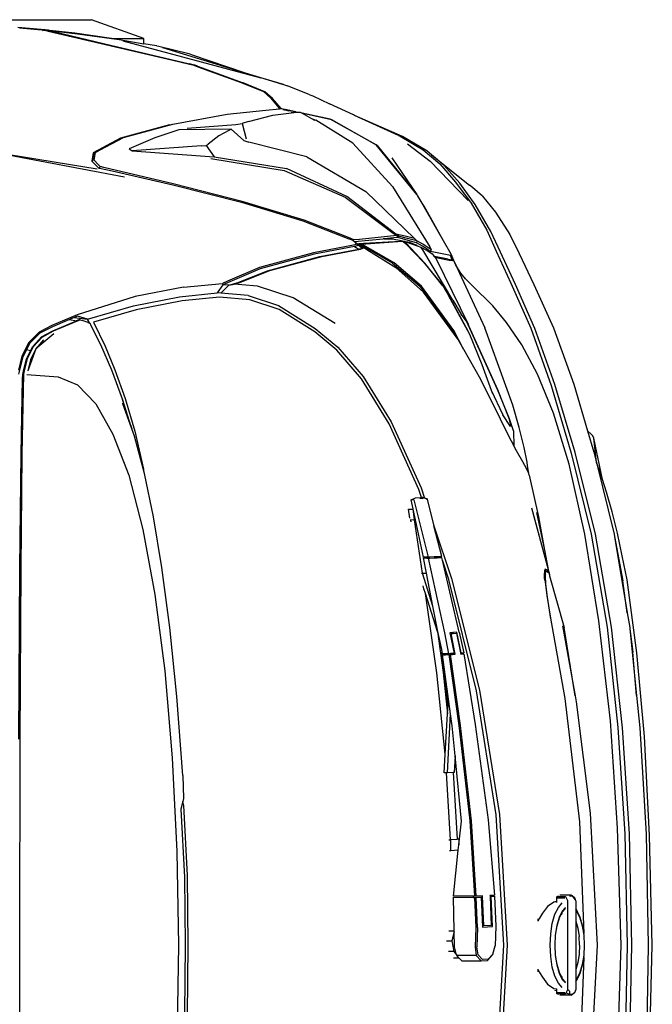
# Model space of a CAD drawing. Units: inches. Extents: x 22042254 to 25404563, y 17568978 to 17626777.
# Tile 9 of 45: x 22042256.4081 to 22042256.7839, y 17568978.1821 to 17568978.767. Entities that reach past the tile are written whole.
import ezdxf

# ---------------------------------------------------------------- set-up
doc = ezdxf.new("R2010")
doc.units = ezdxf.units.IN
doc.header["$MEASUREMENT"] = 0
doc.layers.add('A-SITE-VEHI', color=8, linetype='Continuous', lineweight=18)
doc.layers.add('Edges', color=250, linetype='Continuous')

# ---------------------------------------------------------------- blocks, each defined once
blk = doc.blocks.new('Nissan Qashqai pl')
at = {"layer": 'Edges'}
for p, q in [((11.05972, 12.11965), (11.05938, 11.92208)), ((11.5166, 12.04708), (11.52386, 11.92208)), ((11.52698, 11.92208), (11.51964, 12.0475)), ((11.61327, 11.92208), (11.60675, 12.04892)), ((11.60051, 11.93346), (11.59629, 12.04057)), ((11.63292, 12.0344), (11.63628, 11.92208)), ((11.64211, 11.92208), (11.63993, 12.02899)), ((11.64437, 12.02886), (11.64655, 11.92208)), ((11.66226, 11.92208), (11.66041, 12.02874)), ((11.66349, 12.02738), (11.66628, 11.92208)), ((11.21164, 11.92208), (11.21014, 12.01197)), ((11.22044, 11.98904), (11.22108, 11.92208)), ((11.21801, 11.92208), (11.21745, 11.98742)), ((11.57617, 11.96938), (11.57479, 11.96843)), ((11.58846, 11.97008), (11.57758, 11.97008)), ((11.58668, 11.96947), (11.58377, 11.96782)), ((11.58679, 11.96604), (11.58668, 11.96947)), ((11.58961, 11.96947), (11.58668, 11.96947)), ((11.58846, 11.97008), (11.58961, 11.96947)), ((11.5915, 11.96782), (11.58961, 11.96947)), ((11.56588, 11.95938), (11.57195, 11.96347)), ((11.57195, 11.96347), (11.57457, 11.96395)), ((11.57261, 11.96533), (11.57261, 11.96561)), ((11.57306, 11.96528), (11.57306, 11.96569)), ((11.57479, 11.96843), (11.57457, 11.96768)), ((11.58239, 11.96768), (11.57457, 11.96768)), ((11.57457, 11.96768), (11.57457, 11.96395)), ((11.57457, 11.96395), (11.57457, 11.96378)), ((11.57479, 11.96843), (11.58262, 11.96843)), ((11.57994, 11.96265), (11.57613, 11.95845)), ((11.58262, 11.96843), (11.58377, 11.96782)), ((11.58377, 11.96782), (11.58513, 11.96453)), ((11.58679, 11.96604), (11.58513, 11.96453)), ((11.58513, 11.96453), (11.58513, 11.87963)), ((11.5915, 11.96782), (11.59043, 11.96839)), ((11.59285, 11.96453), (11.5915, 11.96782)), ((11.59285, 11.95694), (11.59285, 11.96453)), ((11.55816, 11.94815), (11.56082, 11.95281)), ((11.56082, 11.95281), (11.56588, 11.95938)), ((11.57286, 11.95178), (11.57035, 11.94308)), ((11.57613, 11.95845), (11.57286, 11.95178)), ((11.57692, 11.94885), (11.57987, 11.95487)), ((11.57876, 11.95169), (11.57712, 11.94834)), ((11.58001, 11.95424), (11.57876, 11.95169)), ((11.57876, 11.95169), (11.57995, 11.953)), ((11.57987, 11.95487), (11.58291, 11.95821)), ((11.58291, 11.95743), (11.58001, 11.95424)), ((11.59285, 11.95694), (11.59412, 11.95487)), ((11.59285, 11.95657), (11.59285, 11.95694)), ((11.59319, 11.9559), (11.59285, 11.95657)), ((11.59285, 11.95626), (11.59285, 11.95657)), ((11.59285, 11.95626), (11.59319, 11.9559)), ((11.59285, 11.95549), (11.59285, 11.95626)), ((11.59398, 11.95424), (11.59285, 11.95549)), ((11.59285, 11.94526), (11.59285, 11.95549)), ((11.59319, 11.9559), (11.59412, 11.95487)), ((11.59688, 11.94834), (11.59398, 11.95424)), ((11.59412, 11.95487), (11.59707, 11.94885)), ((11.55654, 11.94509), (11.55639, 11.94749)), ((11.55654, 11.94509), (11.55816, 11.94815)), ((11.57035, 11.94308), (11.56877, 11.93295)), ((11.57324, 11.93188), (11.57466, 11.94101)), ((11.5749, 11.94065), (11.5735, 11.93169)), ((11.57466, 11.94101), (11.57692, 11.94885)), ((11.57712, 11.94834), (11.5749, 11.94065)), ((11.59285, 11.8989), (11.59285, 11.94526)), ((11.59478, 11.93858), (11.59285, 11.94526)), ((11.5991, 11.94065), (11.59688, 11.94834)), ((11.59707, 11.94885), (11.59933, 11.94101)), ((11.60049, 11.93169), (11.5991, 11.94065)), ((11.59933, 11.94101), (11.60051, 11.93346)), ((11.48106, 11.93457), (11.47554, 11.93456)), ((11.47578, 11.92803), (11.4784, 11.93124)), ((11.4784, 11.93124), (11.47657, 11.92368)), ((11.4786, 11.93206), (11.4784, 11.93124)), ((11.48106, 11.93457), (11.4786, 11.93206)), ((11.49744, 11.93207), (11.4786, 11.93206)), ((11.48349, 11.93703), (11.48106, 11.93457)), ((11.48349, 11.93703), (11.50222, 11.93704)), ((11.49621, 11.92369), (11.49744, 11.93207)), ((11.49744, 11.93207), (11.50222, 11.93704)), ((11.49907, 11.93132), (11.49795, 11.92364)), ((11.50349, 11.93588), (11.49907, 11.93132)), ((11.50222, 11.93704), (11.50812, 11.93671)), ((11.50889, 11.93558), (11.50349, 11.93588)), ((11.50812, 11.93671), (11.51287, 11.9312)), ((11.50889, 11.93558), (11.51321, 11.93053)), ((11.51321, 11.93053), (11.51287, 11.9312)), ((11.56877, 11.93295), (11.56823, 11.92208)), ((11.57275, 11.92208), (11.57324, 11.93188)), ((11.5735, 11.93169), (11.57302, 11.92208)), ((11.59602, 11.93062), (11.59478, 11.93858)), ((11.60097, 11.92208), (11.60049, 11.93169)), ((11.60051, 11.93346), (11.60076, 11.93188)), ((11.60076, 11.93188), (11.60124, 11.92208)), ((11.05938, 11.92208), (11.05972, 11.72451)), ((11.21014, 11.8322), (11.21164, 11.92208)), ((11.21745, 11.85674), (11.21801, 11.92208)), ((11.22108, 11.92208), (11.22044, 11.85512)), ((11.47578, 11.92803), (11.47062, 11.92803)), ((11.47398, 11.91798), (11.47578, 11.92803)), ((11.47657, 11.92368), (11.47622, 11.90912)), ((11.49689, 11.90495), (11.49621, 11.92369)), ((11.49859, 11.9049), (11.49795, 11.92364)), ((11.51321, 11.93053), (11.51543, 11.92267)), ((11.51606, 11.90392), (11.51543, 11.92267)), ((11.52386, 11.92208), (11.5166, 11.79708)), ((11.51964, 11.79666), (11.52698, 11.92208)), ((11.56823, 11.92208), (11.56877, 11.91121)), ((11.57324, 11.91228), (11.57275, 11.92208)), ((11.57302, 11.92208), (11.5735, 11.91247)), ((11.59645, 11.92208), (11.59602, 11.93062)), ((11.59645, 11.92208), (11.59602, 11.91354)), ((11.60049, 11.91247), (11.60097, 11.92208)), ((11.60124, 11.92208), (11.60076, 11.91228)), ((11.60675, 11.79524), (11.61327, 11.92208)), ((11.63628, 11.92208), (11.63292, 11.80976)), ((11.63993, 11.81518), (11.64211, 11.92208)), ((11.64655, 11.92208), (11.64437, 11.8153)), ((11.66041, 11.81542), (11.66226, 11.92208)), ((11.66628, 11.92208), (11.66349, 11.81678)), ((11.46896, 11.91798), (11.47398, 11.91798)), ((11.47622, 11.90912), (11.47398, 11.91798)), ((11.57466, 11.90315), (11.57324, 11.91228)), ((11.5735, 11.91247), (11.5749, 11.90351)), ((11.59478, 11.90558), (11.59602, 11.91354)), ((11.5991, 11.90351), (11.60049, 11.91247)), ((11.60076, 11.91228), (11.60051, 11.91071)), ((11.47102, 11.90825), (11.4762, 11.90826)), ((11.4762, 11.90826), (11.47542, 11.87608)), ((11.47622, 11.90912), (11.4762, 11.90826)), ((11.49565, 11.87616), (11.49689, 11.90495)), ((11.49859, 11.9049), (11.49735, 11.87612)), ((11.50223, 11.8759), (11.50346, 11.90468)), ((11.50462, 11.90341), (11.50341, 11.87505)), ((11.50346, 11.90468), (11.51299, 11.90415)), ((11.51177, 11.90301), (11.50462, 11.90341)), ((11.51058, 11.87508), (11.51177, 11.90301)), ((11.51299, 11.90415), (11.51176, 11.87537)), ((11.51483, 11.87514), (11.51606, 11.90392)), ((11.56877, 11.91121), (11.57035, 11.90108)), ((11.57692, 11.89531), (11.57466, 11.90315)), ((11.5749, 11.90351), (11.57712, 11.89582)), ((11.59285, 11.8989), (11.59478, 11.90558)), ((11.59629, 11.80359), (11.60051, 11.91071)), ((11.59688, 11.89582), (11.5991, 11.90351)), ((11.59933, 11.90315), (11.59707, 11.89531)), ((11.60051, 11.91071), (11.59933, 11.90315)), ((11.55639, 11.89667), (11.55654, 11.89907)), ((11.55816, 11.89601), (11.55654, 11.89907)), ((11.56082, 11.89135), (11.55816, 11.89601)), ((11.57035, 11.90108), (11.57286, 11.89238)), ((11.57987, 11.88929), (11.57692, 11.89531)), ((11.57712, 11.89582), (11.57876, 11.89248)), ((11.59285, 11.88868), (11.59285, 11.8989)), ((11.59398, 11.88992), (11.59688, 11.89582)), ((11.59707, 11.89531), (11.59412, 11.88929)), ((11.56588, 11.88478), (11.56082, 11.89135)), ((11.57195, 11.88069), (11.56588, 11.88478)), ((11.57286, 11.89238), (11.57613, 11.88571)), ((11.57613, 11.88571), (11.57994, 11.88151)), ((11.57995, 11.89116), (11.57876, 11.89248)), ((11.57876, 11.89248), (11.58001, 11.88992)), ((11.58291, 11.88595), (11.57987, 11.88929)), ((11.58001, 11.88992), (11.58291, 11.88673)), ((11.59285, 11.88868), (11.59398, 11.88992)), ((11.59285, 11.88722), (11.59412, 11.88929)), ((11.59285, 11.8879), (11.59285, 11.88868)), ((11.59285, 11.88759), (11.59319, 11.88827)), ((11.59319, 11.88827), (11.59285, 11.8879)), ((11.59285, 11.88759), (11.59285, 11.8879)), ((11.59285, 11.88722), (11.59285, 11.88759)), ((11.59285, 11.87963), (11.59285, 11.88722)), ((11.59412, 11.88929), (11.59319, 11.88827)), ((11.49563, 11.87496), (11.47539, 11.87488)), ((11.47539, 11.87488), (11.4801, 11.83099)), ((11.47542, 11.87608), (11.49451, 11.87616)), ((11.49133, 11.80278), (11.49563, 11.87496)), ((11.49732, 11.87492), (11.49295, 11.80271)), ((11.49449, 11.87502), (11.49451, 11.87616)), ((11.50341, 11.87505), (11.49449, 11.87502)), ((11.49451, 11.87616), (11.49565, 11.87616)), ((11.49732, 11.87492), (11.49563, 11.87496)), ((11.49565, 11.87616), (11.49735, 11.87612)), ((11.50339, 11.87463), (11.49732, 11.87492)), ((11.49735, 11.87612), (11.50223, 11.8759)), ((11.50341, 11.87505), (11.50339, 11.87463)), ((11.51054, 11.87423), (11.51058, 11.87508)), ((11.51472, 11.8751), (11.51058, 11.87508)), ((11.51176, 11.87537), (11.51472, 11.87515)), ((11.51472, 11.87515), (11.51472, 11.8751)), ((11.51472, 11.87515), (11.51483, 11.87514)), ((11.51483, 11.87514), (11.51472, 11.8751)), ((11.57261, 11.88057), (11.57195, 11.88069)), ((11.57261, 11.88057), (11.57261, 11.88076)), ((11.57306, 11.88049), (11.57261, 11.88057)), ((11.57306, 11.88049), (11.57306, 11.88081)), ((11.57457, 11.88021), (11.57306, 11.88049)), ((11.57457, 11.88096), (11.57457, 11.88021)), ((11.57457, 11.88021), (11.57457, 11.87648)), ((11.57457, 11.87648), (11.58239, 11.87648)), ((11.57457, 11.87648), (11.57479, 11.87573)), ((11.58262, 11.87573), (11.57479, 11.87573)), ((11.57479, 11.87573), (11.57617, 11.87478)), ((11.58377, 11.87635), (11.58262, 11.87573)), ((11.58513, 11.87963), (11.58377, 11.87635)), ((11.58668, 11.87469), (11.58961, 11.87469)), ((11.58961, 11.87469), (11.58846, 11.87408)), ((11.58961, 11.87469), (11.5915, 11.87635)), ((11.59043, 11.87577), (11.58961, 11.87469)), ((11.59221, 11.87812), (11.59043, 11.87577)), ((11.59043, 11.87577), (11.5915, 11.87635)), ((11.5915, 11.87635), (11.59221, 11.87812)), ((11.59285, 11.87963), (11.59221, 11.87812)), ((11.50884, 11.80182), (11.5148, 11.87394)), ((11.5148, 11.87394), (11.51054, 11.87423)), ((11.58846, 11.87408), (11.57758, 11.87408)), ((11.2139, 11.7914), (11.21745, 11.85674)), ((11.22044, 11.85512), (11.21682, 11.78816)), ((11.20565, 11.74231), (11.21014, 11.8322)), ((11.47305, 11.83139), (11.47165, 11.83144)), ((11.47305, 11.83139), (11.473, 11.82087)), ((11.4801, 11.83099), (11.47305, 11.83139)), ((11.4801, 11.83099), (11.48065, 11.82584)), ((11.47281, 11.82086), (11.46872, 11.75675)), ((11.47111, 11.82093), (11.47189, 11.82089)), ((11.47281, 11.82086), (11.47189, 11.82089)), ((11.473, 11.82087), (11.47281, 11.82086)), ((11.47916, 11.8205), (11.473, 11.82087)), ((11.47508, 11.75641), (11.47919, 11.82046)), ((11.47919, 11.82046), (11.47916, 11.8205)), ((11.48062, 11.82044), (11.47919, 11.82046)), ((11.48062, 11.82044), (11.48065, 11.82584)), ((11.48065, 11.82584), (11.4831, 11.803)), ((11.63292, 11.80976), (11.62604, 11.70665)), ((11.63327, 11.71316), (11.63993, 11.81518)), ((11.64437, 11.8153), (11.63768, 11.7134)), ((11.65425, 11.71357), (11.66041, 11.81542)), ((11.66349, 11.81678), (11.65888, 11.72193)), ((11.4831, 11.803), (11.47707, 11.74042)), ((11.4805, 11.71128), (11.49133, 11.80278)), ((11.49295, 11.80271), (11.48212, 11.71121)), ((11.49642, 11.71041), (11.50884, 11.80182)), ((11.58235, 11.68521), (11.59629, 11.80359)), ((11.21579, 11.78424), (11.2139, 11.7914)), ((11.5166, 11.79708), (11.49761, 11.67796)), ((11.50045, 11.6772), (11.51964, 11.79666)), ((11.5932, 11.68852), (11.60675, 11.79524)), ((11.21682, 11.78816), (11.21579, 11.78424)), ((11.21585, 11.78401), (11.21579, 11.78424)), ((11.21682, 11.78816), (11.21585, 11.78401)), ((11.21658, 11.78121), (11.21585, 11.78401)), ((11.21586, 11.75915), (11.21658, 11.78121)), ((11.21586, 11.75915), (11.20997, 11.68347)), ((11.46872, 11.75675), (11.46649, 11.75682)), ((11.46649, 11.75682), (11.46757, 11.73891)), ((11.46975, 11.75671), (11.46872, 11.75675)), ((11.46975, 11.75671), (11.47273, 11.69994)), ((11.47508, 11.75641), (11.46975, 11.75671)), ((11.47611, 11.75636), (11.47508, 11.75641)), ((11.47707, 11.74042), (11.47611, 11.75636)), ((11.19842, 11.65867), (11.20565, 11.74231)), ((11.46757, 11.73891), (11.45941, 11.6607)), ((11.46757, 11.73891), (11.46992, 11.70014)), ((11.47707, 11.74042), (11.47428, 11.71144)), ((11.0586, 11.72441), (11.05947, 11.55994)), ((11.05972, 11.72451), (11.06059, 11.56009)), ((11.65888, 11.72193), (11.65143, 11.64152)), ((11.47094, 11.64327), (11.4805, 11.71128)), ((11.48212, 11.71121), (11.47257, 11.6432)), ((11.47428, 11.71144), (11.47273, 11.69994)), ((11.48539, 11.64249), (11.49642, 11.71041)), ((11.62604, 11.70665), (11.61495, 11.61084)), ((11.6229, 11.61679), (11.63327, 11.71316)), ((11.63768, 11.7134), (11.62719, 11.61693)), ((11.65114, 11.68233), (11.65425, 11.71357)), ((11.47273, 11.69994), (11.46512, 11.64343)), ((11.46576, 11.66035), (11.46992, 11.70014)), ((11.46992, 11.70014), (11.47047, 11.69095)), ((11.47047, 11.69095), (11.46419, 11.63849)), ((11.59218, 11.68277), (11.5932, 11.68852)), ((11.20997, 11.68347), (11.2033, 11.61723)), ((11.49761, 11.67796), (11.47115, 11.57128)), ((11.47375, 11.5702), (11.50045, 11.6772)), ((11.56846, 11.60829), (11.58235, 11.68521)), ((11.58021, 11.61555), (11.59218, 11.68277)), ((11.59218, 11.68277), (11.58179, 11.61717)), ((11.64478, 11.61839), (11.65114, 11.68233)), ((11.65114, 11.68233), (11.64749, 11.64092)), ((11.18907, 11.58559), (11.19842, 11.65867)), ((11.45941, 11.6607), (11.44866, 11.58459)), ((11.46024, 11.62121), (11.46576, 11.66035)), ((11.46419, 11.63849), (11.46114, 11.62406)), ((11.46505, 11.64255), (11.46419, 11.63849)), ((11.46792, 11.64248), (11.46505, 11.64255)), ((11.46512, 11.64343), (11.46801, 11.64335)), ((11.46687, 11.62247), (11.47088, 11.64239)), ((11.46801, 11.64335), (11.46792, 11.64248)), ((11.47088, 11.64239), (11.46792, 11.64248)), ((11.46801, 11.64335), (11.47094, 11.64327)), ((11.47252, 11.64233), (11.47088, 11.64239)), ((11.47094, 11.64327), (11.47257, 11.6432)), ((11.47212, 11.62223), (11.47625, 11.64214)), ((11.47439, 11.64223), (11.47252, 11.64233)), ((11.47257, 11.6432), (11.47449, 11.6431)), ((11.47727, 11.64296), (11.47315, 11.62305)), ((11.47439, 11.64223), (11.47449, 11.6431)), ((11.47625, 11.64214), (11.47439, 11.64223)), ((11.47449, 11.6431), (11.47727, 11.64296)), ((11.47827, 11.62277), (11.48226, 11.64167)), ((11.48298, 11.64165), (11.47879, 11.62186)), ((11.48098, 11.62171), (11.48532, 11.64161)), ((11.48226, 11.64167), (11.48244, 11.64254)), ((11.48226, 11.64167), (11.48298, 11.64165)), ((11.48244, 11.64254), (11.48247, 11.64267)), ((11.48535, 11.64246), (11.48244, 11.64254)), ((11.48247, 11.64267), (11.48535, 11.64246)), ((11.483, 11.64176), (11.48298, 11.64165)), ((11.48532, 11.64161), (11.483, 11.64176)), ((11.48539, 11.64249), (11.48535, 11.64246)), ((11.65143, 11.64152), (11.64217, 11.57162)), ((11.64478, 11.61839), (11.64749, 11.64092)), ((11.46024, 11.62121), (11.44866, 11.58459)), ((11.45125, 11.55073), (11.46687, 11.62247)), ((11.46083, 11.62261), (11.45585, 11.5969)), ((11.46114, 11.62406), (11.46024, 11.62121)), ((11.46114, 11.62406), (11.46083, 11.62261)), ((11.48098, 11.62171), (11.4649, 11.55261)), ((11.47495, 11.62207), (11.47212, 11.62223)), ((11.47315, 11.62305), (11.47515, 11.62294)), ((11.47495, 11.62207), (11.47515, 11.62294)), ((11.47879, 11.62186), (11.47495, 11.62207)), ((11.47515, 11.62294), (11.47827, 11.62277)), ((11.2033, 11.61723), (11.19582, 11.55976)), ((11.56776, 11.56755), (11.58179, 11.61717)), ((11.61495, 11.61084), (11.6016, 11.52761)), ((11.60765, 11.5276), (11.6229, 11.61679)), ((11.62719, 11.61693), (11.61178, 11.52762)), ((11.64227, 11.603), (11.64462, 11.61709)), ((11.64462, 11.61709), (11.64478, 11.61839)), ((11.56499, 11.58644), (11.56846, 11.60829)), ((11.56905, 11.60888), (11.56563, 11.58822)), ((11.63012, 11.53004), (11.64227, 11.603)), ((11.64227, 11.603), (11.63807, 11.5726)), ((11.45585, 11.5969), (11.44582, 11.56516)), ((11.45585, 11.5969), (11.44965, 11.56495)), ((11.17758, 11.52307), (11.18907, 11.58559)), ((11.44866, 11.58459), (11.44723, 11.58007)), ((11.56356, 11.57357), (11.56499, 11.58644)), ((11.56563, 11.58822), (11.56415, 11.57536)), ((11.44723, 11.58007), (11.44639, 11.57739)), ((11.56335, 11.56843), (11.56356, 11.57357)), ((11.56415, 11.57536), (11.56375, 11.56794)), ((11.63012, 11.53004), (11.63807, 11.5726)), ((11.44575, 11.56516), (11.43801, 11.51398)), ((11.4448, 11.5652), (11.44575, 11.56516)), ((11.44575, 11.56516), (11.44582, 11.56516)), ((11.44582, 11.56516), (11.44965, 11.56495)), ((11.44965, 11.56495), (11.44685, 11.5505)), ((11.45676, 11.51971), (11.47375, 11.5702)), ((11.47115, 11.57128), (11.4649, 11.55261)), ((11.56255, 11.56701), (11.56268, 11.56956)), ((11.56271, 11.56245), (11.56255, 11.56701)), ((11.56268, 11.56956), (11.56259, 11.5697)), ((11.56268, 11.56956), (11.5628, 11.57206)), ((11.56335, 11.56843), (11.56268, 11.56956)), ((11.56325, 11.56586), (11.56335, 11.56843)), ((11.56334, 11.56271), (11.56325, 11.56586)), ((11.56609, 11.56386), (11.56334, 11.56271)), ((11.56368, 11.56788), (11.56335, 11.56843)), ((11.56375, 11.56794), (11.56392, 11.56325)), ((11.56392, 11.56325), (11.56429, 11.56338)), ((11.56429, 11.56338), (11.56596, 11.56408)), ((11.56487, 11.5659), (11.56469, 11.5662)), ((11.56609, 11.56386), (11.56583, 11.56223)), ((11.56596, 11.56408), (11.56616, 11.56417)), ((11.56609, 11.56386), (11.56596, 11.56408)), ((11.56613, 11.56388), (11.56609, 11.56386)), ((11.56618, 11.56418), (11.56613, 11.56388)), ((11.56613, 11.56388), (11.56616, 11.56417)), ((11.56613, 11.56388), (11.56645, 11.5641)), ((11.56665, 11.56424), (11.56616, 11.56236)), ((11.56616, 11.56417), (11.56618, 11.56418)), ((11.56616, 11.56236), (11.56645, 11.5641)), ((11.56618, 11.56418), (11.56648, 11.56431)), ((11.56645, 11.5641), (11.56648, 11.56431)), ((11.56645, 11.5641), (11.56665, 11.56424)), ((11.56648, 11.56431), (11.56669, 11.5644)), ((11.56661, 11.56253), (11.56704, 11.56455)), ((11.56665, 11.56424), (11.56688, 11.56448)), ((11.56669, 11.5644), (11.56665, 11.56424)), ((11.56669, 11.5644), (11.56688, 11.56448)), ((11.56671, 11.56257), (11.56712, 11.56458)), ((11.56717, 11.5646), (11.56679, 11.56261)), ((11.56688, 11.56448), (11.56704, 11.56455)), ((11.56704, 11.56455), (11.56739, 11.56625)), ((11.56704, 11.56455), (11.56712, 11.56458)), ((11.56712, 11.56458), (11.56763, 11.56708)), ((11.56712, 11.56458), (11.56717, 11.5646)), ((11.56717, 11.5646), (11.56763, 11.56708)), ((11.56745, 11.56646), (11.56739, 11.56625)), ((11.56763, 11.56708), (11.56776, 11.56755)), ((11.64217, 11.57162), (11.63751, 11.54857)), ((11.05947, 11.55994), (11.06074, 11.45082)), ((11.06059, 11.56009), (11.06182, 11.4509)), ((11.19582, 11.55976), (11.18773, 11.51111)), ((11.55053, 11.5023), (11.56648, 11.56144)), ((11.56334, 11.56271), (11.56271, 11.56245)), ((11.56338, 11.56129), (11.56271, 11.56245)), ((11.56273, 11.5431), (11.56648, 11.56144)), ((11.56338, 11.56129), (11.56334, 11.56271)), ((11.56583, 11.56223), (11.56338, 11.56129)), ((11.56616, 11.56236), (11.56583, 11.56223)), ((11.56661, 11.56253), (11.56616, 11.56236)), ((11.56679, 11.56261), (11.56648, 11.56144)), ((11.56671, 11.56257), (11.56661, 11.56253)), ((11.56679, 11.56261), (11.56671, 11.56257)), ((11.43747, 11.49463), (11.45125, 11.54985)), ((11.44684, 11.54963), (11.43914, 11.51392)), ((11.44983, 11.54978), (11.44684, 11.54963)), ((11.44685, 11.5505), (11.44997, 11.55066)), ((11.44983, 11.54978), (11.44997, 11.55066)), ((11.45125, 11.54985), (11.44983, 11.54978)), ((11.44997, 11.55066), (11.45125, 11.55073)), ((11.45125, 11.55073), (11.4529, 11.55066)), ((11.4529, 11.54978), (11.45125, 11.54985)), ((11.4529, 11.55066), (11.45711, 11.55045)), ((11.45711, 11.54958), (11.4529, 11.54978)), ((11.46429, 11.54915), (11.45676, 11.51971)), ((11.45711, 11.55045), (11.45994, 11.5503)), ((11.46197, 11.5493), (11.45711, 11.54958)), ((11.45983, 11.54978), (11.45994, 11.5503)), ((11.46402, 11.54999), (11.45983, 11.54978)), ((11.45994, 11.5503), (11.46197, 11.55018)), ((11.46197, 11.55018), (11.46404, 11.55004)), ((11.46375, 11.54918), (11.46197, 11.5493)), ((11.46402, 11.54999), (11.46375, 11.54918)), ((11.46429, 11.54915), (11.46375, 11.54918)), ((11.46404, 11.55004), (11.46402, 11.54999)), ((11.46423, 11.55), (11.46402, 11.54999)), ((11.46404, 11.55004), (11.46423, 11.55)), ((11.46423, 11.55), (11.46424, 11.55003)), ((11.4643, 11.55002), (11.46423, 11.55)), ((11.4649, 11.55261), (11.4643, 11.55002)), ((11.63751, 11.54857), (11.63276, 11.52672)), ((11.55533, 11.50682), (11.56273, 11.5431)), ((11.55707, 11.51104), (11.56273, 11.5431)), ((11.6016, 11.52761), (11.58664, 11.46068)), ((11.58843, 11.44985), (11.60765, 11.5276)), ((11.61178, 11.52762), (11.59225, 11.44945)), ((11.61272, 11.45895), (11.62966, 11.52759)), ((11.63276, 11.52672), (11.62771, 11.50627)), ((11.62966, 11.52759), (11.63012, 11.53004)), ((11.16395, 11.47112), (11.17758, 11.52307)), ((11.43501, 11.51584), (11.43475, 11.51409)), ((11.45032, 11.49453), (11.45676, 11.51971)), ((11.18773, 11.51111), (11.17906, 11.46956)), ((11.43371, 11.51238), (11.43251, 11.50378)), ((11.43475, 11.51409), (11.43403, 11.51411)), ((11.43801, 11.51398), (11.43475, 11.51409)), ((11.4382, 11.51397), (11.43676, 11.50364)), ((11.43914, 11.51392), (11.43692, 11.50363)), ((11.4382, 11.51397), (11.43801, 11.51398)), ((11.43914, 11.51392), (11.4382, 11.51397)), ((11.54814, 11.47101), (11.55707, 11.51104)), ((11.62771, 11.50627), (11.62241, 11.48743)), ((11.43251, 11.50378), (11.43676, 11.50364)), ((11.43251, 11.50378), (11.4369, 11.50353)), ((11.4369, 11.50353), (11.435, 11.49469)), ((11.43676, 11.50364), (11.43692, 11.50363)), ((11.43692, 11.50363), (11.4369, 11.50353)), ((11.435, 11.49469), (11.43896, 11.49272)), ((11.43747, 11.49463), (11.435, 11.49469)), ((11.43896, 11.49272), (11.44373, 11.49245)), ((11.44474, 11.49242), (11.44218, 11.48476)), ((11.44507, 11.49341), (11.44316, 11.49351)), ((11.44373, 11.49245), (11.44491, 11.49291)), ((11.44474, 11.49242), (11.44373, 11.49245)), ((11.44453, 11.48334), (11.44778, 11.49299)), ((11.44491, 11.49291), (11.44474, 11.49242)), ((11.4462, 11.49239), (11.44474, 11.49242)), ((11.44507, 11.49341), (11.44491, 11.49291)), ((11.44491, 11.49291), (11.44606, 11.49335)), ((11.44606, 11.49335), (11.44507, 11.49341)), ((11.44786, 11.49325), (11.44606, 11.49335)), ((11.44786, 11.49325), (11.4462, 11.49239)), ((11.44778, 11.49299), (11.4462, 11.49239)), ((11.45018, 11.49392), (11.44778, 11.49299)), ((11.44794, 11.49325), (11.44786, 11.49325)), ((11.45032, 11.49453), (11.44794, 11.49325)), ((11.45018, 11.49392), (11.45032, 11.49453)), ((11.62241, 11.48743), (11.61848, 11.47528)), ((11.44218, 11.48476), (11.41383, 11.42186)), ((11.41588, 11.41997), (11.44453, 11.48334)), ((11.14869, 11.43161), (11.16395, 11.47112)), ((11.17906, 11.46956), (11.17808, 11.46592)), ((11.54554, 11.46484), (11.54721, 11.46841)), ((11.54814, 11.47101), (11.54666, 11.46197)), ((11.61848, 11.47528), (11.61008, 11.43562)), ((11.61742, 11.47198), (11.61272, 11.45895)), ((11.61848, 11.47528), (11.61742, 11.47198)), ((11.17808, 11.46592), (11.1694, 11.43374)), ((11.1699, 11.42889), (11.17797, 11.4652)), ((11.17797, 11.4652), (11.17808, 11.46592)), ((11.54162, 11.45783), (11.54554, 11.46484)), ((11.54666, 11.46197), (11.54611, 11.45874)), ((11.58664, 11.46068), (11.57152, 11.41151)), ((11.61272, 11.45895), (11.61008, 11.43562)), ((11.61028, 11.44915), (11.61272, 11.45895)), ((11.06074, 11.45082), (11.06214, 11.37845)), ((11.06182, 11.4509), (11.06324, 11.37414)), ((11.53572, 11.44731), (11.54162, 11.45783)), ((11.54611, 11.45874), (11.54336, 11.44449)), ((11.56912, 11.38501), (11.58843, 11.44985)), ((11.59225, 11.44945), (11.57263, 11.38419)), ((11.52833, 11.43321), (11.53335, 11.4428)), ((11.53261, 11.43965), (11.5333, 11.44225)), ((11.53313, 11.42848), (11.53354, 11.44315)), ((11.5333, 11.44225), (11.53335, 11.4428)), ((11.53335, 11.4428), (11.53354, 11.44315)), ((11.53354, 11.44315), (11.53572, 11.44731)), ((11.54336, 11.44449), (11.53855, 11.42543)), ((11.60419, 11.42861), (11.61028, 11.44915)), ((11.1323, 11.40268), (11.14869, 11.43161)), ((11.1694, 11.43374), (11.1668, 11.42651)), ((11.5202, 11.41712), (11.52833, 11.43321)), ((11.60772, 11.43162), (11.60419, 11.42861)), ((11.60938, 11.43347), (11.60772, 11.43162)), ((11.61008, 11.43562), (11.60938, 11.43347)), ((11.1668, 11.42651), (11.1582, 11.40259)), ((11.16047, 11.39766), (11.1699, 11.42889)), ((11.16426, 11.41918), (11.1668, 11.42651)), ((11.41383, 11.42186), (11.38718, 11.37878)), ((11.53009, 11.42439), (11.52299, 11.41307)), ((11.52855, 11.41625), (11.53022, 11.42324)), ((11.53313, 11.42848), (11.52922, 11.417)), ((11.53022, 11.42324), (11.53009, 11.42439)), ((11.53855, 11.42543), (11.53253, 11.4038)), ((11.59084, 11.38361), (11.60419, 11.42861)), ((11.15764, 11.39828), (11.16426, 11.41918)), ((11.15766, 11.39771), (11.16426, 11.41918)), ((11.16426, 11.41918), (11.15826, 11.40186)), ((11.38877, 11.37638), (11.41588, 11.41997)), ((11.50131, 11.37908), (11.5202, 11.41712)), ((11.5118, 11.38938), (11.52299, 11.41307)), ((11.52922, 11.417), (11.51787, 11.38901)), ((11.51787, 11.38901), (11.52855, 11.41625)), ((11.11477, 11.38434), (11.1323, 11.40268)), ((11.53253, 11.4038), (11.50574, 11.32965)), ((11.57152, 11.41151), (11.55624, 11.37411)), ((11.14751, 11.37001), (11.15766, 11.39771)), ((11.15051, 11.36998), (11.16047, 11.39766)), ((11.5118, 11.38938), (11.51304, 11.39274)), ((11.09618, 11.37663), (11.11477, 11.38434)), ((11.51787, 11.38901), (11.48801, 11.32337)), ((11.49005, 11.3275), (11.51787, 11.38901)), ((11.50277, 11.36495), (11.5118, 11.38938)), ((11.54963, 11.33002), (11.56912, 11.38501)), ((11.57263, 11.38419), (11.5535, 11.33028)), ((11.57164, 11.32969), (11.59084, 11.38361)), ((11.06236, 11.3576), (11.05822, 11.37418)), ((11.06214, 11.37845), (11.06222, 11.37449)), ((11.06222, 11.37449), (11.06303, 11.37135)), ((11.06324, 11.37414), (11.06408, 11.37085)), ((11.06624, 11.37435), (11.09618, 11.37663)), ((11.38718, 11.37878), (11.3635, 11.35125)), ((11.36451, 11.34835), (11.38877, 11.37638)), ((11.48518, 11.35017), (11.50131, 11.37908)), ((11.55624, 11.37411), (11.54097, 11.34593)), ((11.06139, 11.35691), (11.05807, 11.37037)), ((11.06303, 11.37135), (11.06594, 11.3594)), ((11.06408, 11.37085), (11.06692, 11.35921)), ((11.06961, 11.36056), (11.0671, 11.37109)), ((11.07472, 11.34981), (11.0671, 11.37109)), ((11.13692, 11.34555), (11.14751, 11.37001)), ((11.14123, 11.34726), (11.15051, 11.36998)), ((11.49086, 11.33567), (11.50277, 11.36495)), ((11.06818, 11.34377), (11.06139, 11.35691)), ((11.06584, 11.35092), (11.06236, 11.3576)), ((11.06594, 11.3594), (11.06978, 11.35164)), ((11.06692, 11.35921), (11.0727, 11.34754)), ((11.07472, 11.34981), (11.06961, 11.36056)), ((11.06978, 11.35164), (11.06584, 11.35092)), ((11.06918, 11.34452), (11.06584, 11.35092)), ((11.06978, 11.35164), (11.07183, 11.3475)), ((11.07183, 11.3475), (11.08018, 11.33842)), ((11.0727, 11.34754), (11.0809, 11.33858)), ((11.08206, 11.34125), (11.07472, 11.34981)), ((11.092, 11.33548), (11.07472, 11.34981)), ((11.12767, 11.32749), (11.13692, 11.34555)), ((11.13017, 11.32416), (11.14123, 11.34726)), ((11.3635, 11.35125), (11.34251, 11.3336)), ((11.34283, 11.33026), (11.36451, 11.34835)), ((11.48518, 11.35017), (11.4758, 11.33232)), ((11.48012, 11.34111), (11.48518, 11.35017)), ((11.54097, 11.34593), (11.52646, 11.32473)), ((11.07787, 11.3339), (11.06818, 11.34377)), ((11.07866, 11.33492), (11.06918, 11.34452)), ((11.08018, 11.33842), (11.09121, 11.33249)), ((11.0809, 11.33858), (11.09174, 11.33271)), ((11.48005, 11.341), (11.44669, 11.29536)), ((11.47876, 11.33901), (11.47454, 11.33252)), ((11.47876, 11.33901), (11.48005, 11.341)), ((11.48005, 11.341), (11.48012, 11.34111)), ((11.09022, 11.32753), (11.07787, 11.3339)), ((11.09081, 11.32882), (11.07866, 11.33492)), ((11.11439, 11.31711), (11.09022, 11.32753)), ((11.10704, 11.32181), (11.09081, 11.32882)), ((11.09121, 11.33249), (11.1138, 11.3229)), ((11.09174, 11.33271), (11.11486, 11.323)), ((11.12645, 11.32495), (11.12767, 11.32749)), ((11.30757, 11.30833), (11.34283, 11.33026)), ((11.34251, 11.3336), (11.3082, 11.31215)), ((11.44331, 11.28988), (11.47454, 11.33252)), ((11.4758, 11.33232), (11.44474, 11.28965)), ((11.46332, 11.28473), (11.48966, 11.33337)), ((11.47038, 11.29841), (11.49086, 11.33567)), ((11.47038, 11.29841), (11.48966, 11.33337)), ((11.48133, 11.27727), (11.50574, 11.32965)), ((11.48983, 11.32694), (11.48954, 11.32636)), ((11.48966, 11.33337), (11.49086, 11.33567)), ((11.48983, 11.32694), (11.49005, 11.3275)), ((11.53062, 11.28691), (11.54963, 11.33002)), ((11.5535, 11.33028), (11.53487, 11.28826)), ((11.55274, 11.28821), (11.57164, 11.32969)), ((11.10704, 11.32181), (11.1138, 11.3229)), ((11.11164, 11.31982), (11.10704, 11.32181)), ((11.11164, 11.31982), (11.1244, 11.32146)), ((11.11467, 11.31851), (11.11164, 11.31982)), ((11.1138, 11.3229), (11.11393, 11.32284)), ((11.11393, 11.32284), (11.1164, 11.32172)), ((11.1244, 11.32146), (11.11467, 11.31851)), ((11.11486, 11.323), (11.1172, 11.32196)), ((11.1164, 11.32172), (11.1172, 11.32196)), ((11.11744, 11.32189), (11.1164, 11.32172)), ((11.1172, 11.32196), (11.11744, 11.32189)), ((11.11744, 11.32189), (11.11997, 11.32267)), ((11.11997, 11.32267), (11.12459, 11.32429)), ((11.12604, 11.32481), (11.1244, 11.32146)), ((11.1244, 11.32146), (11.12591, 11.32476)), ((11.1244, 11.32146), (11.16836, 11.30873)), ((11.12459, 11.32429), (11.12591, 11.32476)), ((11.12466, 11.32442), (11.12595, 11.32486)), ((11.12478, 11.32467), (11.12595, 11.32486)), ((11.12595, 11.32486), (11.1251, 11.3253)), ((11.12591, 11.32476), (11.12595, 11.32486)), ((11.12591, 11.32476), (11.12604, 11.32481)), ((11.12595, 11.32486), (11.12626, 11.32554)), ((11.12595, 11.32486), (11.12607, 11.32488)), ((11.12604, 11.32481), (11.12645, 11.32495)), ((11.12607, 11.32488), (11.12604, 11.32481)), ((11.12631, 11.32537), (11.12607, 11.32488)), ((11.12607, 11.32488), (11.12645, 11.32495)), ((11.17121, 11.31245), (11.13017, 11.32416)), ((11.36192, 11.32544), (11.32179, 11.30083)), ((11.45883, 11.26345), (11.48954, 11.32636)), ((11.48801, 11.32337), (11.48281, 11.31653)), ((11.52646, 11.32473), (11.51313, 11.30854)), ((11.17021, 11.29978), (11.11439, 11.31711)), ((11.16836, 11.30873), (11.21271, 11.29983)), ((11.21523, 11.3038), (11.17121, 11.31245)), ((11.27848, 11.29865), (11.30757, 11.30833)), ((11.3082, 11.31215), (11.28005, 11.30276)), ((11.47499, 11.30324), (11.48281, 11.31653)), ((11.51313, 11.30854), (11.49329, 11.28912)), ((11.21656, 11.2908), (11.17021, 11.29978)), ((11.21271, 11.29983), (11.24875, 11.29618)), ((11.2509, 11.3003), (11.21523, 11.3038)), ((11.28005, 11.30276), (11.2509, 11.3003)), ((11.27848, 11.29865), (11.25238, 11.29648)), ((11.32179, 11.30083), (11.28736, 11.28974)), ((11.47499, 11.30324), (11.4462, 11.25482)), ((11.47026, 11.29821), (11.47038, 11.29841)), ((11.21656, 11.2908), (11.25377, 11.28706)), ((11.25238, 11.29648), (11.24875, 11.29618)), ((11.2541, 11.28846), (11.24875, 11.29618)), ((11.25238, 11.29648), (11.25993, 11.28891)), ((11.25993, 11.28891), (11.2541, 11.28846)), ((11.25993, 11.28891), (11.25999, 11.28889)), ((11.25999, 11.28889), (11.26503, 11.28789)), ((11.25999, 11.28889), (11.26771, 11.28668)), ((11.28736, 11.28974), (11.27242, 11.28847)), ((11.41708, 11.26758), (11.44331, 11.28988)), ((11.44474, 11.28965), (11.41866, 11.26734)), ((11.42028, 11.27173), (11.44669, 11.29536)), ((11.44691, 11.26684), (11.46587, 11.29022)), ((11.46538, 11.28932), (11.44788, 11.2676)), ((11.46538, 11.28932), (11.46587, 11.29022)), ((11.46587, 11.29022), (11.46737, 11.29293)), ((11.46746, 11.29312), (11.46737, 11.29293)), ((11.46746, 11.29312), (11.47026, 11.29821)), ((11.49329, 11.28912), (11.48692, 11.28262)), ((11.25857, 11.28503), (11.25377, 11.28706)), ((11.29, 11.2731), (11.2541, 11.28846)), ((11.28951, 11.27177), (11.25857, 11.28503)), ((11.27242, 11.28847), (11.26503, 11.28789)), ((11.26503, 11.28789), (11.27055, 11.28622)), ((11.26771, 11.28668), (11.26785, 11.28663)), ((11.26785, 11.28663), (11.29721, 11.27493)), ((11.27055, 11.28622), (11.29928, 11.27468)), ((11.48692, 11.28262), (11.48256, 11.27724)), ((11.51652, 11.25601), (11.53062, 11.28691)), ((11.53487, 11.28826), (11.52058, 11.25724)), ((11.53843, 11.2583), (11.55274, 11.28821)), ((11.3411, 11.25789), (11.28951, 11.27177)), ((11.34188, 11.25916), (11.29, 11.2731)), ((11.29721, 11.27493), (11.34742, 11.26142)), ((11.29928, 11.27468), (11.34932, 11.2614)), ((11.39234, 11.25471), (11.42028, 11.27173)), ((11.47707, 11.26812), (11.48133, 11.27727)), ((11.48256, 11.27724), (11.47783, 11.26953)), ((11.48133, 11.27727), (11.48217, 11.27864)), ((11.34742, 11.26142), (11.38475, 11.2543)), ((11.34932, 11.2614), (11.38634, 11.25437)), ((11.41708, 11.26758), (11.38507, 11.24911)), ((11.41866, 11.26734), (11.3914, 11.25156)), ((11.42958, 11.2488), (11.44691, 11.26684)), ((11.44788, 11.2676), (11.43028, 11.24852)), ((11.45491, 11.25868), (11.45678, 11.26054)), ((11.4564, 11.26086), (11.45669, 11.26088)), ((11.45652, 11.26104), (11.45688, 11.26111)), ((11.45678, 11.26054), (11.45714, 11.2609)), ((11.45714, 11.2609), (11.45732, 11.2612)), ((11.45729, 11.26188), (11.45734, 11.2619)), ((11.47041, 11.26385), (11.45732, 11.2612)), ((11.45732, 11.2612), (11.45781, 11.262)), ((11.45736, 11.26195), (11.45734, 11.2619)), ((11.45736, 11.26195), (11.45755, 11.26195)), ((11.45781, 11.262), (11.45883, 11.26345)), ((11.45781, 11.262), (11.46047, 11.26254)), ((11.46047, 11.26254), (11.46049, 11.26254)), ((11.46049, 11.26254), (11.47129, 11.26473)), ((11.47041, 11.26385), (11.47423, 11.26446)), ((11.47129, 11.26473), (11.47442, 11.26498)), ((11.47463, 11.26457), (11.47278, 11.2604)), ((11.47423, 11.26446), (11.47278, 11.2604)), ((11.47281, 11.2603), (11.47317, 11.26096)), ((11.47585, 11.26509), (11.47322, 11.2592)), ((11.47423, 11.26446), (11.47445, 11.26449)), ((11.47442, 11.26498), (11.47433, 11.26475)), ((11.47442, 11.26498), (11.47446, 11.26498)), ((11.47445, 11.26477), (11.47446, 11.26498)), ((11.47463, 11.26457), (11.47445, 11.26449)), ((11.47446, 11.26498), (11.47482, 11.26501)), ((11.47585, 11.26509), (11.47463, 11.26457)), ((11.47482, 11.26501), (11.47475, 11.26484)), ((11.47482, 11.26501), (11.47585, 11.26509)), ((11.47588, 11.26517), (11.47585, 11.26509)), ((11.47783, 11.26953), (11.47588, 11.26517)), ((11.47707, 11.26812), (11.47588, 11.26517)), ((11.37955, 11.25028), (11.3411, 11.25789)), ((11.38043, 11.25154), (11.34188, 11.25916)), ((11.38043, 11.25154), (11.38475, 11.2543)), ((11.38408, 11.25081), (11.38043, 11.25154)), ((11.38295, 11.24897), (11.38801, 11.25321)), ((11.38475, 11.2543), (11.38801, 11.25321)), ((11.38823, 11.2519), (11.38491, 11.2491)), ((11.38811, 11.25194), (11.3861, 11.25078)), ((11.38634, 11.25437), (11.38953, 11.25299)), ((11.3914, 11.25156), (11.3867, 11.24922)), ((11.38862, 11.25223), (11.38822, 11.252)), ((11.38862, 11.25223), (11.38823, 11.2519)), ((11.39063, 11.25338), (11.38862, 11.25223)), ((11.38953, 11.25299), (11.38862, 11.25223)), ((11.38953, 11.25299), (11.39234, 11.25471)), ((11.41698, 11.19425), (11.45295, 11.25195)), ((11.44573, 11.25131), (11.43996, 11.24823)), ((11.44061, 11.25095), (11.44418, 11.2522)), ((11.44418, 11.2522), (11.44968, 11.25519)), ((11.4462, 11.25482), (11.44418, 11.2522)), ((11.45121, 11.25489), (11.44573, 11.25131)), ((11.45199, 11.25317), (11.44624, 11.24948)), ((11.44968, 11.25519), (11.44984, 11.25529)), ((11.44984, 11.25529), (11.45491, 11.25868)), ((11.44984, 11.25529), (11.45351, 11.25651)), ((11.45121, 11.25489), (11.45351, 11.25651)), ((11.45386, 11.25448), (11.45199, 11.25317)), ((11.45295, 11.25195), (11.45421, 11.25473)), ((11.45316, 11.25595), (11.45351, 11.25651)), ((11.47278, 11.2604), (11.45351, 11.25651)), ((11.45351, 11.25651), (11.45421, 11.25473)), ((11.45421, 11.25473), (11.45386, 11.25448)), ((11.47322, 11.2592), (11.46579, 11.24614)), ((11.47197, 11.25711), (11.47177, 11.25676)), ((11.47269, 11.26007), (11.47281, 11.2603)), ((11.47278, 11.2604), (11.47281, 11.2603)), ((11.47281, 11.2603), (11.47322, 11.2592)), ((11.50736, 11.23616), (11.51652, 11.25601)), ((11.52058, 11.25724), (11.51126, 11.23721)), ((11.52949, 11.24004), (11.53843, 11.2583)), ((11.33108, 11.22699), (11.37506, 11.24429)), ((11.37475, 11.24309), (11.33228, 11.22637)), ((11.38, 11.24532), (11.37475, 11.24309)), ((11.37506, 11.24429), (11.37524, 11.24436)), ((11.37506, 11.24429), (11.37621, 11.24429)), ((11.37922, 11.24593), (11.37524, 11.24436)), ((11.3763, 11.24436), (11.37524, 11.24436)), ((11.37922, 11.24593), (11.38041, 11.24692)), ((11.37933, 11.24631), (11.37922, 11.24593)), ((11.38338, 11.24949), (11.37955, 11.25028)), ((11.38533, 11.24487), (11.38, 11.24532)), ((11.38041, 11.24692), (11.38275, 11.24887)), ((11.38041, 11.24692), (11.40818, 11.24436)), ((11.38129, 11.24847), (11.38167, 11.2488)), ((11.38275, 11.24887), (11.38338, 11.24949)), ((11.38446, 11.24984), (11.38295, 11.24897)), ((11.38295, 11.24897), (11.38491, 11.2491)), ((11.38295, 11.24897), (11.38461, 11.24885)), ((11.38408, 11.25081), (11.38338, 11.24949)), ((11.38461, 11.24885), (11.38464, 11.24887)), ((11.38461, 11.24885), (11.38934, 11.2486)), ((11.38464, 11.24887), (11.38501, 11.24911)), ((11.38491, 11.2491), (11.38464, 11.24887)), ((11.38501, 11.24911), (11.38507, 11.24911)), ((11.38507, 11.24911), (11.3867, 11.24922)), ((11.42115, 11.24117), (11.38533, 11.24487)), ((11.3867, 11.24922), (11.3915, 11.24906)), ((11.38934, 11.2486), (11.42481, 11.24653)), ((11.3915, 11.24906), (11.42659, 11.2465)), ((11.3915, 11.19885), (11.4381, 11.24397)), ((11.41644, 11.24436), (11.40818, 11.24436)), ((11.40898, 11.24429), (11.40818, 11.24436)), ((11.40898, 11.24429), (11.4163, 11.24429)), ((11.4152, 11.24371), (11.40898, 11.24429)), ((11.4163, 11.24429), (11.4152, 11.24371)), ((11.42154, 11.24313), (11.4152, 11.24371)), ((11.41644, 11.24436), (11.4163, 11.24429)), ((11.41686, 11.24458), (11.41644, 11.24436)), ((11.4252, 11.2462), (11.41686, 11.24458)), ((11.42915, 11.24177), (11.42033, 11.23975)), ((11.42287, 11.24164), (11.42033, 11.23975)), ((11.42115, 11.24117), (11.42154, 11.24313)), ((11.42296, 11.24352), (11.42154, 11.24313)), ((11.42287, 11.24164), (11.42178, 11.24134)), ((11.43154, 11.24397), (11.42287, 11.24164)), ((11.42296, 11.24352), (11.42287, 11.24164)), ((11.43996, 11.24823), (11.42296, 11.24352)), ((11.42481, 11.24653), (11.42659, 11.2465)), ((11.42659, 11.2465), (11.4252, 11.2462)), ((11.42659, 11.2465), (11.42684, 11.24649)), ((11.42684, 11.24649), (11.42958, 11.2488)), ((11.42684, 11.24649), (11.42784, 11.24647)), ((11.43028, 11.24852), (11.42784, 11.24647)), ((11.42784, 11.24647), (11.42996, 11.24721)), ((11.4381, 11.24397), (11.42915, 11.24177)), ((11.42996, 11.24721), (11.43609, 11.24937)), ((11.43368, 11.248), (11.42996, 11.24721)), ((11.44027, 11.24637), (11.43154, 11.24397)), ((11.4397, 11.25049), (11.43368, 11.248)), ((11.43609, 11.24937), (11.44061, 11.25095)), ((11.4381, 11.24397), (11.44027, 11.24637)), ((11.44061, 11.25095), (11.4397, 11.25049)), ((11.44027, 11.24637), (11.43996, 11.24823)), ((11.44624, 11.24948), (11.44027, 11.24637)), ((11.44114, 11.20281), (11.46562, 11.24583)), ((11.44697, 11.21272), (11.46562, 11.24583)), ((11.46562, 11.24583), (11.46579, 11.24614)), ((11.3715, 11.20434), (11.41772, 11.23895)), ((11.42033, 11.23975), (11.37334, 11.20375)), ((11.41772, 11.23895), (11.41931, 11.23998)), ((11.41915, 11.23969), (11.4194, 11.23996)), ((11.41931, 11.23998), (11.4196, 11.24017)), ((11.4194, 11.23996), (11.41931, 11.23998)), ((11.4194, 11.23996), (11.4196, 11.24017)), ((11.41958, 11.23992), (11.4194, 11.23996)), ((11.4196, 11.24017), (11.42014, 11.24052)), ((11.41984, 11.24006), (11.42014, 11.24052)), ((11.42014, 11.24052), (11.42115, 11.24117)), ((11.42178, 11.24134), (11.42115, 11.24117)), ((11.42216, 11.24127), (11.42178, 11.24134)), ((11.49236, 11.21027), (11.50736, 11.23616)), ((11.51126, 11.23721), (11.49628, 11.21137)), ((11.51576, 11.21859), (11.52949, 11.24004)), ((11.27199, 11.20923), (11.33108, 11.22699)), ((11.33228, 11.22637), (11.27276, 11.20843)), ((11.50327, 11.20341), (11.51576, 11.21859)), ((11.20627, 11.19262), (11.27199, 11.20923)), ((11.27276, 11.20843), (11.20665, 11.19145)), ((11.31316, 11.17892), (11.3715, 11.20434)), ((11.44697, 11.21272), (11.44114, 11.20281)), ((11.45306, 11.16974), (11.48975, 11.20767)), ((11.47745, 11.18983), (11.49236, 11.21027)), ((11.49628, 11.21137), (11.48154, 11.19102)), ((11.37334, 11.20375), (11.31527, 11.17691)), ((11.33497, 11.16556), (11.3915, 11.19885)), ((11.44046, 11.20182), (11.40144, 11.15414)), ((11.40216, 11.15476), (11.44046, 11.20182)), ((11.41633, 11.16662), (11.44046, 11.20182)), ((11.44081, 11.20225), (11.44046, 11.20182)), ((11.4411, 11.20277), (11.44081, 11.20225)), ((11.44114, 11.20281), (11.4411, 11.20277)), ((11.49363, 11.19502), (11.49082, 11.19282)), ((11.50327, 11.20341), (11.49363, 11.19502)), ((11.20665, 11.19145), (11.14012, 11.17593)), ((11.14803, 11.17913), (11.20627, 11.19262)), ((11.37896, 11.15265), (11.41698, 11.19425)), ((11.45433, 11.16358), (11.49082, 11.19282)), ((11.46237, 11.17248), (11.47745, 11.18983)), ((11.48154, 11.19102), (11.46617, 11.17358)), ((11.03575, 11.16129), (11.1598, 11.18473)), ((11.04919, 11.16347), (11.13359, 11.17719)), ((11.12929, 11.17052), (11.13526, 11.17642)), ((11.13526, 11.17642), (11.13585, 11.17654)), ((11.13585, 11.17654), (11.14803, 11.17913)), ((11.13585, 11.17654), (11.13658, 11.17502)), ((11.14012, 11.17593), (11.13658, 11.17502)), ((11.24278, 11.16729), (11.31316, 11.17892)), ((11.24587, 11.16563), (11.31527, 11.17691)), ((11.12846, 11.16971), (11.12929, 11.17052)), ((11.12977, 11.16183), (11.12846, 11.16971)), ((11.12929, 11.17052), (11.13057, 11.16299)), ((11.1347, 11.17313), (11.13062, 11.16899)), ((11.13062, 11.16899), (11.13192, 11.16144)), ((11.13658, 11.17502), (11.1347, 11.17313)), ((11.43143, 11.15309), (11.45306, 11.16974)), ((11.44642, 11.15882), (11.46237, 11.17248)), ((11.46617, 11.17358), (11.45433, 11.16358)), ((11.15597, 11.14759), (11.12977, 11.16183)), ((11.13192, 11.16144), (11.13057, 11.16299)), ((11.13192, 11.16144), (11.13652, 11.15905)), ((11.13652, 11.15905), (11.15893, 11.14704)), ((11.16444, 11.15792), (11.16717, 11.15976)), ((11.18896, 11.14734), (11.16444, 11.15792)), ((11.16717, 11.15976), (11.24587, 11.16563)), ((11.23369, 11.15498), (11.16717, 11.15976)), ((11.23823, 11.15494), (11.24587, 11.16563)), ((11.33497, 11.16556), (11.27913, 11.15147)), ((11.42433, 11.14593), (11.44642, 11.15882)), ((11.44983, 11.15977), (11.42671, 11.14629)), ((11.45433, 11.16358), (11.44983, 11.15977)), ((11.20291, 11.13489), (11.15597, 11.14759)), ((11.2121, 11.1399), (11.18896, 11.14734)), ((11.23369, 11.15498), (11.23823, 11.15494)), ((11.23823, 11.15494), (11.2401, 11.15337)), ((11.25046, 11.1455), (11.2401, 11.15337)), ((11.27429, 11.14993), (11.26224, 11.13901)), ((11.27289, 11.13379), (11.27664, 11.14845)), ((11.27429, 11.14993), (11.27913, 11.15147)), ((11.37896, 11.15265), (11.34336, 11.13032)), ((11.40144, 11.15414), (11.3571, 11.12956)), ((11.35832, 11.12998), (11.40144, 11.15414)), ((11.40216, 11.15476), (11.40144, 11.15414)), ((11.15893, 11.14704), (11.20616, 11.13437)), ((11.26224, 11.13901), (11.2121, 11.1399)), ((11.21991, 11.1382), (11.26663, 11.13449)), ((11.26005, 11.1405), (11.25046, 11.1455)), ((11.26224, 11.13901), (11.26005, 11.1405)), ((11.42671, 11.14629), (11.38067, 11.12595)), ((11.42283, 11.14525), (11.38067, 11.12595)), ((11.42283, 11.14525), (11.42433, 11.14593)), ((11.20291, 11.13489), (11.20295, 11.13488)), ((11.20295, 11.13488), (11.20616, 11.13437)), ((11.20616, 11.13437), (11.25827, 11.12461)), ((11.26663, 11.13449), (11.27289, 11.13379)), ((11.27871, 11.13184), (11.27289, 11.13379)), ((11.27871, 11.13184), (11.30218, 11.1256)), ((11.32955, 11.12347), (11.3571, 11.12956)), ((11.3571, 11.12956), (11.33021, 11.12384)), ((11.33021, 11.12384), (11.33938, 11.12898)), ((11.33938, 11.12898), (11.34202, 11.13045)), ((11.33938, 11.12898), (11.34336, 11.13032)), ((11.3571, 11.12956), (11.35832, 11.12998)), ((11.25827, 11.12461), (11.29558, 11.12077)), ((11.29558, 11.12077), (11.30849, 11.1195)), ((11.30003, 11.10916), (11.30813, 11.11883)), ((11.31027, 11.11923), (11.30178, 11.10961)), ((11.30218, 11.1256), (11.32517, 11.12286)), ((11.30805, 11.11884), (11.30863, 11.11948)), ((11.30813, 11.11883), (11.30863, 11.11948)), ((11.30849, 11.1195), (11.30863, 11.11948)), ((11.30863, 11.11948), (11.31033, 11.1193)), ((11.31033, 11.1193), (11.31027, 11.11923)), ((11.31033, 11.1193), (11.31061, 11.11927)), ((11.31061, 11.11927), (11.314, 11.12039)), ((11.31704, 11.12142), (11.31186, 11.12058)), ((11.31323, 11.11986), (11.32588, 11.12266)), ((11.32423, 11.12258), (11.314, 11.12039)), ((11.314, 11.12039), (11.31704, 11.12142)), ((11.32423, 11.12258), (11.31704, 11.12142)), ((11.31982, 11.1231), (11.32517, 11.12286)), ((11.32423, 11.12258), (11.32588, 11.12266)), ((11.32517, 11.12286), (11.32831, 11.12278)), ((11.32588, 11.12266), (11.32831, 11.12278)), ((11.32831, 11.12278), (11.32955, 11.12347)), ((11.32955, 11.12347), (11.33021, 11.12384)), ((11.37962, 11.12547), (11.35656, 11.11477)), ((11.38067, 11.12595), (11.37962, 11.12547)), ((11.30178, 11.10961), (11.29459, 11.10327)), ((11.34052, 11.10725), (11.35656, 11.11477)), ((11.29459, 11.10327), (11.27358, 11.0947)), ((11.27407, 11.09522), (11.29339, 11.10313)), ((11.29339, 11.10313), (11.30003, 11.10916)), ((11.33757, 11.10603), (11.31612, 11.09747)), ((11.33757, 11.10603), (11.34052, 11.10725)), ((11.2732, 11.09452), (11.22772, 11.07792)), ((11.23038, 11.07923), (11.27187, 11.09432)), ((11.27187, 11.09432), (11.27407, 11.09522)), ((11.27358, 11.0947), (11.2732, 11.09452)), ((11.27358, 11.0947), (11.27407, 11.09522)), ((11.27568, 11.08503), (11.31244, 11.09628)), ((11.31244, 11.09628), (11.29065, 11.08989)), ((11.30801, 11.09508), (11.30877, 11.09528)), ((11.31244, 11.09628), (11.31612, 11.09747)), ((11.15816, 11.05423), (11.29065, 11.08989)), ((11.19633, 11.06072), (11.27568, 11.08503)), ((11.22475, 11.06772), (11.27568, 11.08503)), ((11.08649, 11.04496), (11.21998, 11.07614)), ((11.22216, 11.0766), (11.08821, 11.045)), ((11.09177, 11.04531), (11.22216, 11.0766)), ((11.21998, 11.07614), (11.22216, 11.0766)), ((11.2222, 11.07656), (11.22216, 11.0766)), ((11.22715, 11.07771), (11.2222, 11.07656)), ((11.22238, 11.07665), (11.2222, 11.07656)), ((11.22238, 11.07665), (11.22532, 11.07737)), ((11.22532, 11.07737), (11.23038, 11.07923)), ((11.22731, 11.07783), (11.22706, 11.07777)), ((11.22962, 11.07837), (11.22715, 11.07771)), ((11.22772, 11.07792), (11.22715, 11.07771)), ((11.22962, 11.07837), (11.22772, 11.07792)), ((11.19297, 11.05964), (11.22148, 11.06662)), ((11.22148, 11.06662), (11.22475, 11.06772)), ((11.11474, 11.04762), (11.15472, 11.05317)), ((11.15248, 11.05278), (11.14751, 11.05208)), ((11.15472, 11.05317), (11.15248, 11.05278)), ((11.15472, 11.05317), (11.17828, 11.05716)), ((11.19065, 11.05923), (11.17828, 11.05716)), ((11.17828, 11.05716), (11.17828, 11.05208)), ((11.19089, 11.05929), (11.19065, 11.05923)), ((11.19089, 11.05929), (11.19297, 11.05964)), ((11.07977, 11.04339), (11.05762, 11.04159)), ((11.05899, 11.04188), (11.07681, 11.04337)), ((11.07681, 11.04337), (11.08106, 11.04371)), ((11.08696, 11.04422), (11.07977, 11.04339)), ((11.08106, 11.04371), (11.08273, 11.0441)), ((11.08114, 11.04436), (11.08208, 11.0442)), ((11.08273, 11.0441), (11.08562, 11.04476)), ((11.08273, 11.0441), (11.08365, 11.04395)), ((11.08821, 11.045), (11.08365, 11.04395)), ((11.08365, 11.04395), (11.08696, 11.04422)), ((11.08562, 11.04476), (11.08649, 11.04496)), ((11.08649, 11.04496), (11.08796, 11.04514)), ((11.08696, 11.04422), (11.08721, 11.04424)), ((11.08728, 11.04426), (11.08721, 11.04424)), ((11.08728, 11.04426), (11.08834, 11.04438)), ((11.08834, 11.04438), (11.11474, 11.04762)), ((11.11234, 11.04716), (11.08834, 11.04438)), ((11.14751, 11.05208), (11.11234, 11.04716)), ((11.17828, 11.05208), (11.12828, 11.03408)), ((11.14751, 11.05208), (11.17828, 11.05208)), ((10.95773, 11.03408), (11.12828, 11.03408))]:
    blk.add_line(p, q, dxfattribs=at)
blk = doc.blocks.new('CAR')
blk.add_blockref('Nissan Qashqai pl', (-9.74328, -11.91512))

msp = doc.modelspace()

# ---------------------------------------------------------------- block references
at = {"layer": 'A-SITE-VEHI', "xscale": -0.6191396643141144, "yscale": 0.6191396643141144, "zscale": 0.6191396643141144, "rotation": 180}
msp.add_blockref('CAR', (22042255.59333, 17568978.22147), dxfattribs=at)

doc.saveas('drawing.dxf')
